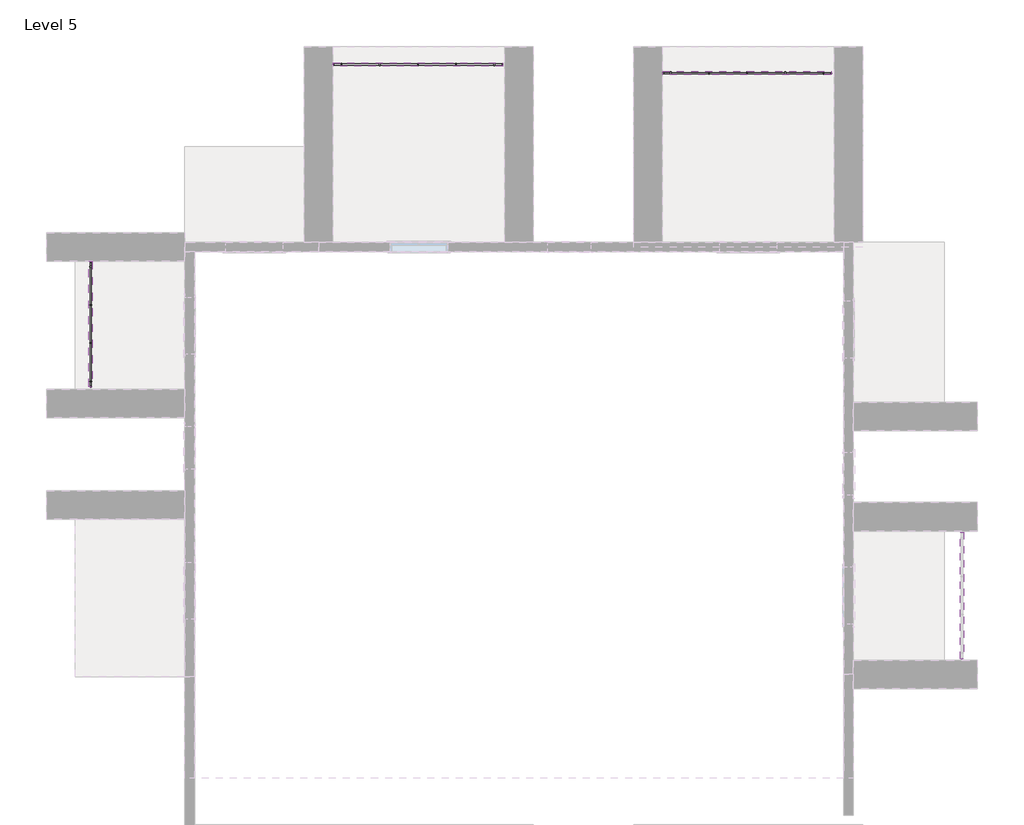
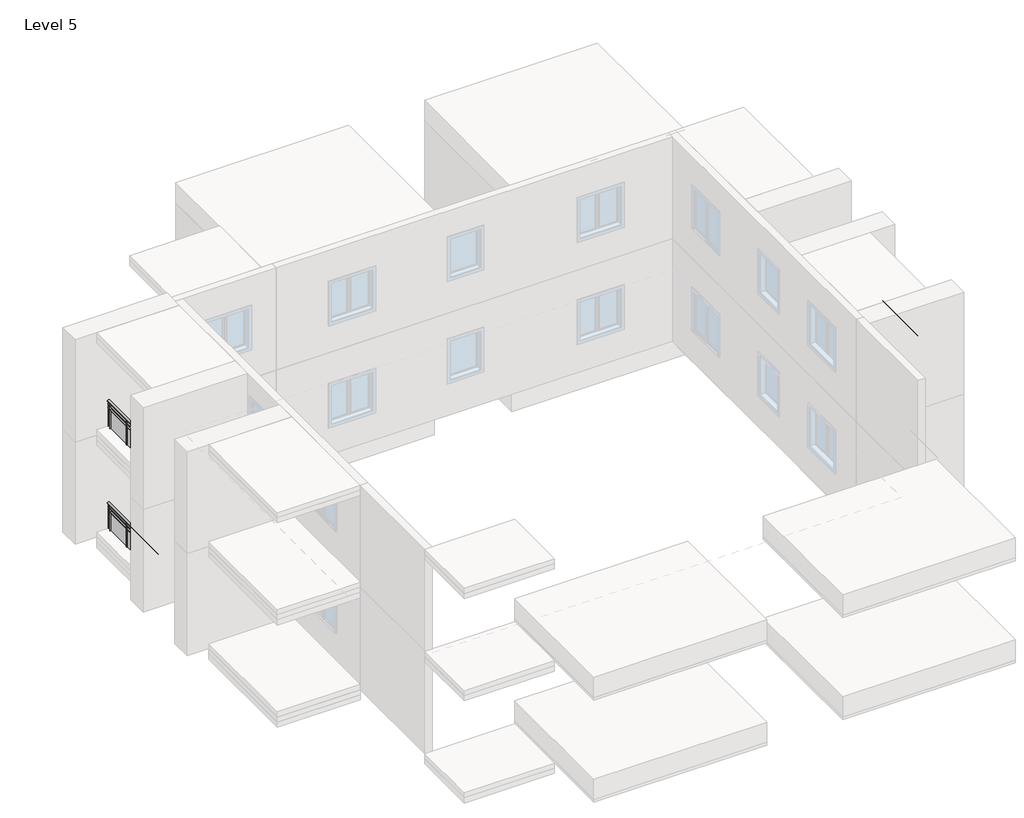
# One storey, part 4 of 4: 7 railings.
"""IFC4 building model written with IfcOpenShell, lengths in millimetres."""

from ifc_helpers import new_model, si_unit, point, frame, origin, place, context, project, spatial, polyline, ellipse_curve, trimmed, outline, extrude, element, save
from ifc_brep_helpers import plane_surface, extruded_surface, advanced_brep

model = new_model("IFC4")

# Units and contexts
model_context = context("Model", 3, world=origin())
ifc_project = project(units=[si_unit("LENGTHUNIT", "METRE", prefix="MILLI")], contexts=[model_context])

# Site, building, storey
site = spatial("IfcSite", under=ifc_project)
building = spatial("IfcBuilding", under=site)
storey = spatial("IfcBuildingStorey", under=building, Name="Level 5", Elevation=12192.0)

# Railings
placement = place(None, origin())
element("IfcRailing", 1, ObjectType="Glass Panel - Bottom Fill", at=placement, inside=storey, context=model_context, shape_type="SolidModel", body=[
    advanced_brep(
    [(-14351.1937431, 6115.813611, 13411.2), (-14427.3937431, 6115.813611, 13411.2), (-14351.1937431, 3448.813611, 13411.2), (-14427.3937431, 3448.813611, 13411.2)],
    [
        (0, 1, ellipse_curve(frame((-14389.2937431, 6115.813611, 13411.2), z_axis=(0.0, 1.0, 0.0), x_axis=(-1.0, 0.0, 0.0)), 38.1, 28.575)),
        (1, 0, ellipse_curve(frame((-14389.2937431, 6115.813611, 13411.2), z_axis=(0.0, 1.0, 0.0), x_axis=(-1.0, 0.0, 0.0)), 38.1, 28.575)),
        (2, 3, ellipse_curve(frame((-14389.2937431, 3448.813611, 13411.2), z_axis=(0.0, -1.0, 0.0), x_axis=(-1.0, 0.0, 0.0)), 38.1, 28.575)),
        (3, 2, ellipse_curve(frame((-14389.2937431, 3448.813611, 13411.2), z_axis=(0.0, -1.0, 0.0), x_axis=(-1.0, 0.0, 0.0)), 38.1, 28.575)),
        (0, 2),
        (3, 1),
    ],
    [
        plane_surface(frame((-14389.2937431, 6115.813611, 13411.2), z_axis=(0.0, 1.0, 0.0), x_axis=(0.0, 0.0, -1.0))),
        plane_surface(frame((-14389.2937431, 3448.813611, 13411.2), z_axis=(0.0, -1.0, 0.0), x_axis=(0.0, 0.0, -1.0))),
        extruded_surface(trimmed(ellipse_curve(frame((-14389.2937431, 3448.813611, 13411.2), z_axis=(0.0, 1.0, 0.0), x_axis=(-1.0, 0.0, 0.0)), 38.1, 28.575), [point((-14351.1937431, 3448.813611, 13411.2))], [point((-14427.3937431, 3448.813611, 13411.2))], True, "CARTESIAN"), (0.0, 2666.9999999999995, 0.0), 2666.9999999999995),
        extruded_surface(trimmed(ellipse_curve(frame((-14389.2937431, 3448.813611, 13411.2), z_axis=(0.0, 1.0, 0.0), x_axis=(-1.0, 0.0, 0.0)), 38.1, 28.575), [point((-14427.3937431, 3448.813611, 13411.2))], [point((-14351.1937431, 3448.813611, 13411.2))], True, "CARTESIAN"), (0.0, 2666.9999999999995, 0.0), 2666.9999999999995),
    ],
    [
        (0, [[1, 2]]),
        (1, [[3, 4]]),
        (2, [[-1, 5, -4, 6]]),
        (3, [[-2, -6, -3, -5]]),
    ],
),
    extrude(outline(polyline([(-14401.9937431, 6115.813611), (-14376.5937431, 6115.813611), (-14376.5937431, 3448.813611), (-14401.9937431, 3448.813611), (-14401.9937431, 6115.813611)])), frame((0.0, 0.0, 13296.9), z_axis=(0.0, 0.0, 1.0), x_axis=(1.0, 0.0, 0.0)), (0.0, 0.0, 1.0), 25.4),
    extrude(outline(polyline([(-14401.9937431, 6115.813611), (-14376.5937431, 6115.813611), (-14376.5937431, 3448.813611), (-14401.9937431, 3448.813611), (-14401.9937431, 6115.813611)])), frame((0.0, 0.0, 13195.3), z_axis=(0.0, 0.0, 1.0), x_axis=(1.0, 0.0, 0.0)), (0.0, 0.0, 1.0), 25.4),
    extrude(outline(polyline([(-14414.6937431, 3569.463611), (-14363.8937431, 3569.463611), (-14363.8937431, 3556.763611), (-14414.6937431, 3556.763611), (-14414.6937431, 3569.463611)])), frame((0.0, 0.0, 12496.8), z_axis=(0.0, 0.0, 1.0), x_axis=(1.0, 0.0, 0.0)), (0.0, 0.0, 1.0), 885.6788223),
    extrude(outline(polyline([(-14382.7585861, 4375.913611), (-14382.7585861, 3563.113611), (-14389.1085861, 3563.113611), (-14389.1085861, 4375.913611), (-14382.7585861, 4375.913611)])), frame((0.0, 0.0, 12598.4), z_axis=(0.0, 0.0, 1.0), x_axis=(1.0, 0.0, 0.0)), (0.0, 0.0, 1.0), 596.9),
    extrude(outline(polyline([(-14414.6937431, 4382.263611), (-14363.8937431, 4382.263611), (-14363.8937431, 4369.563611), (-14414.6937431, 4369.563611), (-14414.6937431, 4382.263611)])), frame((0.0, 0.0, 12496.8), z_axis=(0.0, 0.0, 1.0), x_axis=(1.0, 0.0, 0.0)), (0.0, 0.0, 1.0), 885.6788223),
    extrude(outline(polyline([(-14382.7585861, 5188.713611), (-14382.7585861, 4375.913611), (-14389.1085861, 4375.913611), (-14389.1085861, 5188.713611), (-14382.7585861, 5188.713611)])), frame((0.0, 0.0, 12598.4), z_axis=(0.0, 0.0, 1.0), x_axis=(1.0, 0.0, 0.0)), (0.0, 0.0, 1.0), 596.9),
    extrude(outline(polyline([(-14414.6937431, 5195.063611), (-14363.8937431, 5195.063611), (-14363.8937431, 5182.363611), (-14414.6937431, 5182.363611), (-14414.6937431, 5195.063611)])), frame((0.0, 0.0, 12496.8), z_axis=(0.0, 0.0, 1.0), x_axis=(1.0, 0.0, 0.0)), (0.0, 0.0, 1.0), 885.6788223),
    extrude(outline(polyline([(-14382.7585861, 6001.513611), (-14382.7585861, 5188.713611), (-14389.1085861, 5188.713611), (-14389.1085861, 6001.513611), (-14382.7585861, 6001.513611)])), frame((0.0, 0.0, 12598.4), z_axis=(0.0, 0.0, 1.0), x_axis=(1.0, 0.0, 0.0)), (0.0, 0.0, 1.0), 596.9),
    extrude(outline(polyline([(-14414.6937431, 6007.863611), (-14363.8937431, 6007.863611), (-14363.8937431, 5995.163611), (-14414.6937431, 5995.163611), (-14414.6937431, 6007.863611)])), frame((0.0, 0.0, 12496.8), z_axis=(0.0, 0.0, 1.0), x_axis=(1.0, 0.0, 0.0)), (0.0, 0.0, 1.0), 885.6788223),
    extrude(outline(polyline([(-14398.8187431, 3461.513611), (-14379.7687431, 3461.513611), (-14379.7687431, 3442.463611), (-14398.8187431, 3442.463611), (-14398.8187431, 3461.513611)])), frame((0.0, 0.0, 12496.8), z_axis=(0.0, 0.0, 1.0), x_axis=(1.0, 0.0, 0.0)), (0.0, 0.0, 1.0), 885.6788223),
    extrude(outline(polyline([(-14398.8187431, 6122.163611), (-14379.7687431, 6122.163611), (-14379.7687431, 6103.113611), (-14398.8187431, 6103.113611), (-14398.8187431, 6122.163611)])), frame((0.0, 0.0, 12496.8), z_axis=(0.0, 0.0, 1.0), x_axis=(1.0, 0.0, 0.0)), (0.0, 0.0, 1.0), 885.6788223),
])
element("IfcRailing", 2, ObjectType="Glass Panel - Bottom Fill", at=placement, inside=storey, context=model_context, shape_type="SolidModel", body=[
    advanced_brep(
    [(-9229.0758442, 10344.5205237, 13411.2), (-9229.0758442, 10268.3205237, 13411.2), (-5622.2758442, 10344.5205237, 13411.2), (-5622.2758442, 10268.3205237, 13411.2)],
    [
        (0, 1, ellipse_curve(frame((-9229.0758442, 10306.4205237, 13411.2), z_axis=(-1.0, 0.0, 0.0), x_axis=(0.0, -1.0, 0.0)), 38.1, 28.575)),
        (1, 0, ellipse_curve(frame((-9229.0758442, 10306.4205237, 13411.2), z_axis=(-1.0, 0.0, 0.0), x_axis=(0.0, -1.0, 0.0)), 38.1, 28.575)),
        (2, 3, ellipse_curve(frame((-5622.2758442, 10306.4205237, 13411.2), z_axis=(1.0, 0.0, 0.0), x_axis=(0.0, -1.0, 0.0)), 38.1, 28.575)),
        (3, 2, ellipse_curve(frame((-5622.2758442, 10306.4205237, 13411.2), z_axis=(1.0, 0.0, 0.0), x_axis=(0.0, -1.0, 0.0)), 38.1, 28.575)),
        (0, 2),
        (3, 1),
    ],
    [
        plane_surface(frame((-9229.0758442, 10306.4205237, 13411.2), z_axis=(-1.0, 0.0, 0.0), x_axis=(0.0, 1.0, 0.0))),
        plane_surface(frame((-5622.2758442, 10306.4205237, 13411.2), z_axis=(1.0, 0.0, 0.0), x_axis=(0.0, 1.0, 0.0))),
        extruded_surface(trimmed(ellipse_curve(frame((-5622.2758442, 10306.4205237, 13411.2), z_axis=(-1.0, 0.0, 0.0), x_axis=(0.0, -1.0, 0.0)), 38.1, 28.575), [point((-5622.2758442, 10344.5205237, 13411.2))], [point((-5622.2758442, 10268.3205237, 13411.2))], True, "CARTESIAN"), (-3606.8, 0.0, 0.0), 3606.8),
        extruded_surface(trimmed(ellipse_curve(frame((-5622.2758442, 10306.4205237, 13411.2), z_axis=(-1.0, 0.0, 0.0), x_axis=(0.0, -1.0, 0.0)), 38.1, 28.575), [point((-5622.2758442, 10268.3205237, 13411.2))], [point((-5622.2758442, 10344.5205237, 13411.2))], True, "CARTESIAN"), (-3606.8, 0.0, 0.0), 3606.8),
    ],
    [
        (0, [[1, 2]]),
        (1, [[3, 4]]),
        (2, [[-1, 5, -4, 6]]),
        (3, [[-2, -6, -3, -5]]),
    ],
),
    extrude(outline(polyline([(-9229.0758442, 10293.7205237), (-9229.0758442, 10319.1205237), (-5622.2758442, 10319.1205237), (-5622.2758442, 10293.7205237), (-9229.0758442, 10293.7205237)])), frame((0.0, 0.0, 13296.9), z_axis=(0.0, 0.0, 1.0), x_axis=(1.0, 0.0, 0.0)), (0.0, 0.0, 1.0), 25.4),
    extrude(outline(polyline([(-9229.0758442, 10293.7205237), (-9229.0758442, 10319.1205237), (-5622.2758442, 10319.1205237), (-5622.2758442, 10293.7205237), (-9229.0758442, 10293.7205237)])), frame((0.0, 0.0, 13195.3), z_axis=(0.0, 0.0, 1.0), x_axis=(1.0, 0.0, 0.0)), (0.0, 0.0, 1.0), 25.4),
    extrude(outline(polyline([(-5806.4258442, 10281.0205237), (-5806.4258442, 10331.8205237), (-5793.7258442, 10331.8205237), (-5793.7258442, 10281.0205237), (-5806.4258442, 10281.0205237)])), frame((0.0, 0.0, 12496.8), z_axis=(0.0, 0.0, 1.0), x_axis=(1.0, 0.0, 0.0)), (0.0, 0.0, 1.0), 885.6788223),
    extrude(outline(polyline([(-6612.8758442, 10312.9556807), (-5800.0758442, 10312.9556807), (-5800.0758442, 10306.6056807), (-6612.8758442, 10306.6056807), (-6612.8758442, 10312.9556807)])), frame((0.0, 0.0, 12598.4), z_axis=(0.0, 0.0, 1.0), x_axis=(1.0, 0.0, 0.0)), (0.0, 0.0, 1.0), 596.9),
    extrude(outline(polyline([(-6619.2258442, 10281.0205237), (-6619.2258442, 10331.8205237), (-6606.5258442, 10331.8205237), (-6606.5258442, 10281.0205237), (-6619.2258442, 10281.0205237)])), frame((0.0, 0.0, 12496.8), z_axis=(0.0, 0.0, 1.0), x_axis=(1.0, 0.0, 0.0)), (0.0, 0.0, 1.0), 885.6788223),
    extrude(outline(polyline([(-7425.6758442, 10312.9556807), (-6612.8758442, 10312.9556807), (-6612.8758442, 10306.6056807), (-7425.6758442, 10306.6056807), (-7425.6758442, 10312.9556807)])), frame((0.0, 0.0, 12598.4), z_axis=(0.0, 0.0, 1.0), x_axis=(1.0, 0.0, 0.0)), (0.0, 0.0, 1.0), 596.9),
    extrude(outline(polyline([(-7432.0258442, 10281.0205237), (-7432.0258442, 10331.8205237), (-7419.3258442, 10331.8205237), (-7419.3258442, 10281.0205237), (-7432.0258442, 10281.0205237)])), frame((0.0, 0.0, 12496.8), z_axis=(0.0, 0.0, 1.0), x_axis=(1.0, 0.0, 0.0)), (0.0, 0.0, 1.0), 885.6788223),
    extrude(outline(polyline([(-8238.4758442, 10312.9556807), (-7425.6758442, 10312.9556807), (-7425.6758442, 10306.6056807), (-8238.4758442, 10306.6056807), (-8238.4758442, 10312.9556807)])), frame((0.0, 0.0, 12598.4), z_axis=(0.0, 0.0, 1.0), x_axis=(1.0, 0.0, 0.0)), (0.0, 0.0, 1.0), 596.9),
    extrude(outline(polyline([(-8244.8258442, 10281.0205237), (-8244.8258442, 10331.8205237), (-8232.1258442, 10331.8205237), (-8232.1258442, 10281.0205237), (-8244.8258442, 10281.0205237)])), frame((0.0, 0.0, 12496.8), z_axis=(0.0, 0.0, 1.0), x_axis=(1.0, 0.0, 0.0)), (0.0, 0.0, 1.0), 885.6788223),
    extrude(outline(polyline([(-9051.2758442, 10312.9556807), (-8238.4758442, 10312.9556807), (-8238.4758442, 10306.6056807), (-9051.2758442, 10306.6056807), (-9051.2758442, 10312.9556807)])), frame((0.0, 0.0, 12598.4), z_axis=(0.0, 0.0, 1.0), x_axis=(1.0, 0.0, 0.0)), (0.0, 0.0, 1.0), 596.9),
    extrude(outline(polyline([(-9057.6258442, 10281.0205237), (-9057.6258442, 10331.8205237), (-9044.9258442, 10331.8205237), (-9044.9258442, 10281.0205237), (-9057.6258442, 10281.0205237)])), frame((0.0, 0.0, 12496.8), z_axis=(0.0, 0.0, 1.0), x_axis=(1.0, 0.0, 0.0)), (0.0, 0.0, 1.0), 885.6788223),
    extrude(outline(polyline([(-5634.9758442, 10296.8955237), (-5634.9758442, 10315.9455237), (-5615.9258442, 10315.9455237), (-5615.9258442, 10296.8955237), (-5634.9758442, 10296.8955237)])), frame((0.0, 0.0, 12496.8), z_axis=(0.0, 0.0, 1.0), x_axis=(1.0, 0.0, 0.0)), (0.0, 0.0, 1.0), 885.6788223),
    extrude(outline(polyline([(-9235.4258442, 10296.8955237), (-9235.4258442, 10315.9455237), (-9216.3758442, 10315.9455237), (-9216.3758442, 10296.8955237), (-9235.4258442, 10296.8955237)])), frame((0.0, 0.0, 12496.8), z_axis=(0.0, 0.0, 1.0), x_axis=(1.0, 0.0, 0.0)), (0.0, 0.0, 1.0), 885.6788223),
])
element("IfcRailing", 3, ObjectType="Glass Panel - Bottom Fill", at=placement, inside=storey, context=model_context, shape_type="SolidModel", body=[
    advanced_brep(
    [(-2210.3891352, 10161.3373193, 13411.2), (-2210.3891352, 10085.1373193, 13411.2), (1371.0108648, 10161.3373193, 13411.2), (1371.0108648, 10085.1373193, 13411.2)],
    [
        (0, 1, ellipse_curve(frame((-2210.3891352, 10123.2373193, 13411.2), z_axis=(-1.0, 0.0, 0.0), x_axis=(0.0, -1.0, 0.0)), 38.1, 28.575)),
        (1, 0, ellipse_curve(frame((-2210.3891352, 10123.2373193, 13411.2), z_axis=(-1.0, 0.0, 0.0), x_axis=(0.0, -1.0, 0.0)), 38.1, 28.575)),
        (2, 3, ellipse_curve(frame((1371.0108648, 10123.2373193, 13411.2), z_axis=(1.0, 0.0, 0.0), x_axis=(0.0, -1.0, 0.0)), 38.1, 28.575)),
        (3, 2, ellipse_curve(frame((1371.0108648, 10123.2373193, 13411.2), z_axis=(1.0, 0.0, 0.0), x_axis=(0.0, -1.0, 0.0)), 38.1, 28.575)),
        (0, 2),
        (3, 1),
    ],
    [
        plane_surface(frame((-2210.3891352, 10123.2373193, 13411.2), z_axis=(-1.0, 0.0, 0.0), x_axis=(0.0, 1.0, 0.0))),
        plane_surface(frame((1371.0108648, 10123.2373193, 13411.2), z_axis=(1.0, 0.0, 0.0), x_axis=(0.0, 1.0, 0.0))),
        extruded_surface(trimmed(ellipse_curve(frame((1371.0108648, 10123.2373193, 13411.2), z_axis=(-1.0, 0.0, 0.0), x_axis=(0.0, -1.0, 0.0)), 38.1, 28.575), [point((1371.0108648, 10161.3373193, 13411.2))], [point((1371.0108648, 10085.1373193, 13411.2))], True, "CARTESIAN"), (-3581.4, 0.0, 0.0), 3581.4),
        extruded_surface(trimmed(ellipse_curve(frame((1371.0108648, 10123.2373193, 13411.2), z_axis=(-1.0, 0.0, 0.0), x_axis=(0.0, -1.0, 0.0)), 38.1, 28.575), [point((1371.0108648, 10085.1373193, 13411.2))], [point((1371.0108648, 10161.3373193, 13411.2))], True, "CARTESIAN"), (-3581.4, 0.0, 0.0), 3581.4),
    ],
    [
        (0, [[1, 2]]),
        (1, [[3, 4]]),
        (2, [[-1, 5, -4, 6]]),
        (3, [[-2, -6, -3, -5]]),
    ],
),
    extrude(outline(polyline([(-2210.3891352, 10110.5373193), (-2210.3891352, 10135.9373193), (1371.0108648, 10135.9373193), (1371.0108648, 10110.5373193), (-2210.3891352, 10110.5373193)])), frame((0.0, 0.0, 13296.9), z_axis=(0.0, 0.0, 1.0), x_axis=(1.0, 0.0, 0.0)), (0.0, 0.0, 1.0), 25.4),
    extrude(outline(polyline([(-2210.3891352, 10110.5373193), (-2210.3891352, 10135.9373193), (1371.0108648, 10135.9373193), (1371.0108648, 10110.5373193), (-2210.3891352, 10110.5373193)])), frame((0.0, 0.0, 13195.3), z_axis=(0.0, 0.0, 1.0), x_axis=(1.0, 0.0, 0.0)), (0.0, 0.0, 1.0), 25.4),
    extrude(outline(polyline([(1199.5608648, 10097.8373193), (1199.5608648, 10148.6373193), (1212.2608648, 10148.6373193), (1212.2608648, 10097.8373193), (1199.5608648, 10097.8373193)])), frame((0.0, 0.0, 12496.8), z_axis=(0.0, 0.0, 1.0), x_axis=(1.0, 0.0, 0.0)), (0.0, 0.0, 1.0), 885.6788223),
    extrude(outline(polyline([(393.1108648, 10129.7724763), (1205.9108648, 10129.7724763), (1205.9108648, 10123.4224763), (393.1108648, 10123.4224763), (393.1108648, 10129.7724763)])), frame((0.0, 0.0, 12598.4), z_axis=(0.0, 0.0, 1.0), x_axis=(1.0, 0.0, 0.0)), (0.0, 0.0, 1.0), 596.9),
    extrude(outline(polyline([(386.7608648, 10097.8373193), (386.7608648, 10148.6373193), (399.4608648, 10148.6373193), (399.4608648, 10097.8373193), (386.7608648, 10097.8373193)])), frame((0.0, 0.0, 12496.8), z_axis=(0.0, 0.0, 1.0), x_axis=(1.0, 0.0, 0.0)), (0.0, 0.0, 1.0), 885.6788223),
    extrude(outline(polyline([(-419.6891352, 10129.7724763), (393.1108648, 10129.7724763), (393.1108648, 10123.4224763), (-419.6891352, 10123.4224763), (-419.6891352, 10129.7724763)])), frame((0.0, 0.0, 12598.4), z_axis=(0.0, 0.0, 1.0), x_axis=(1.0, 0.0, 0.0)), (0.0, 0.0, 1.0), 596.9),
    extrude(outline(polyline([(-426.0391352, 10097.8373193), (-426.0391352, 10148.6373193), (-413.3391352, 10148.6373193), (-413.3391352, 10097.8373193), (-426.0391352, 10097.8373193)])), frame((0.0, 0.0, 12496.8), z_axis=(0.0, 0.0, 1.0), x_axis=(1.0, 0.0, 0.0)), (0.0, 0.0, 1.0), 885.6788223),
    extrude(outline(polyline([(-1232.4891352, 10129.7724763), (-419.6891352, 10129.7724763), (-419.6891352, 10123.4224763), (-1232.4891352, 10123.4224763), (-1232.4891352, 10129.7724763)])), frame((0.0, 0.0, 12598.4), z_axis=(0.0, 0.0, 1.0), x_axis=(1.0, 0.0, 0.0)), (0.0, 0.0, 1.0), 596.9),
    extrude(outline(polyline([(-1238.8391352, 10097.8373193), (-1238.8391352, 10148.6373193), (-1226.1391352, 10148.6373193), (-1226.1391352, 10097.8373193), (-1238.8391352, 10097.8373193)])), frame((0.0, 0.0, 12496.8), z_axis=(0.0, 0.0, 1.0), x_axis=(1.0, 0.0, 0.0)), (0.0, 0.0, 1.0), 885.6788223),
    extrude(outline(polyline([(-2045.2891352, 10129.7724763), (-1232.4891352, 10129.7724763), (-1232.4891352, 10123.4224763), (-2045.2891352, 10123.4224763), (-2045.2891352, 10129.7724763)])), frame((0.0, 0.0, 12598.4), z_axis=(0.0, 0.0, 1.0), x_axis=(1.0, 0.0, 0.0)), (0.0, 0.0, 1.0), 596.9),
    extrude(outline(polyline([(-2051.6391352, 10097.8373193), (-2051.6391352, 10148.6373193), (-2038.9391352, 10148.6373193), (-2038.9391352, 10097.8373193), (-2051.6391352, 10097.8373193)])), frame((0.0, 0.0, 12496.8), z_axis=(0.0, 0.0, 1.0), x_axis=(1.0, 0.0, 0.0)), (0.0, 0.0, 1.0), 885.6788223),
    extrude(outline(polyline([(1358.3108648, 10113.7123193), (1358.3108648, 10132.7623193), (1377.3608648, 10132.7623193), (1377.3608648, 10113.7123193), (1358.3108648, 10113.7123193)])), frame((0.0, 0.0, 12496.8), z_axis=(0.0, 0.0, 1.0), x_axis=(1.0, 0.0, 0.0)), (0.0, 0.0, 1.0), 885.6788223),
    extrude(outline(polyline([(-2216.7391352, 10113.7123193), (-2216.7391352, 10132.7623193), (-2197.6891352, 10132.7623193), (-2197.6891352, 10113.7123193), (-2216.7391352, 10113.7123193)])), frame((0.0, 0.0, 12496.8), z_axis=(0.0, 0.0, 1.0), x_axis=(1.0, 0.0, 0.0)), (0.0, 0.0, 1.0), 885.6788223),
])
element("IfcRailing", 4, ObjectType="Glass Panel - Bottom Fill", at=placement, inside=storey, context=model_context, shape_type="SolidModel", body=[
    advanced_brep(
    [(-14351.1937431, 6115.813611, 16459.2), (-14427.3937431, 6115.813611, 16459.2), (-14351.1937431, 3448.813611, 16459.2), (-14427.3937431, 3448.813611, 16459.2)],
    [
        (0, 1, ellipse_curve(frame((-14389.2937431, 6115.813611, 16459.2), z_axis=(0.0, 1.0, 0.0), x_axis=(-1.0, 0.0, 0.0)), 38.1, 28.575)),
        (1, 0, ellipse_curve(frame((-14389.2937431, 6115.813611, 16459.2), z_axis=(0.0, 1.0, 0.0), x_axis=(-1.0, 0.0, 0.0)), 38.1, 28.575)),
        (2, 3, ellipse_curve(frame((-14389.2937431, 3448.813611, 16459.2), z_axis=(0.0, -1.0, 0.0), x_axis=(-1.0, 0.0, 0.0)), 38.1, 28.575)),
        (3, 2, ellipse_curve(frame((-14389.2937431, 3448.813611, 16459.2), z_axis=(0.0, -1.0, 0.0), x_axis=(-1.0, 0.0, 0.0)), 38.1, 28.575)),
        (0, 2),
        (3, 1),
    ],
    [
        plane_surface(frame((-14389.2937431, 6115.813611, 16459.2), z_axis=(0.0, 1.0, 0.0), x_axis=(0.0, 0.0, -1.0))),
        plane_surface(frame((-14389.2937431, 3448.813611, 16459.2), z_axis=(0.0, -1.0, 0.0), x_axis=(0.0, 0.0, -1.0))),
        extruded_surface(trimmed(ellipse_curve(frame((-14389.2937431, 3448.813611, 16459.2), z_axis=(0.0, 1.0, 0.0), x_axis=(-1.0, 0.0, 0.0)), 38.1, 28.575), [point((-14351.1937431, 3448.813611, 16459.2))], [point((-14427.3937431, 3448.813611, 16459.2))], True, "CARTESIAN"), (0.0, 2666.9999999999995, 0.0), 2666.9999999999995),
        extruded_surface(trimmed(ellipse_curve(frame((-14389.2937431, 3448.813611, 16459.2), z_axis=(0.0, 1.0, 0.0), x_axis=(-1.0, 0.0, 0.0)), 38.1, 28.575), [point((-14427.3937431, 3448.813611, 16459.2))], [point((-14351.1937431, 3448.813611, 16459.2))], True, "CARTESIAN"), (0.0, 2666.9999999999995, 0.0), 2666.9999999999995),
    ],
    [
        (0, [[1, 2]]),
        (1, [[3, 4]]),
        (2, [[-1, 5, -4, 6]]),
        (3, [[-2, -6, -3, -5]]),
    ],
),
    extrude(outline(polyline([(-14401.9937431, 6115.813611), (-14376.5937431, 6115.813611), (-14376.5937431, 3448.813611), (-14401.9937431, 3448.813611), (-14401.9937431, 6115.813611)])), frame((0.0, 0.0, 16344.9), z_axis=(0.0, 0.0, 1.0), x_axis=(1.0, 0.0, 0.0)), (0.0, 0.0, 1.0), 25.4),
    extrude(outline(polyline([(-14401.9937431, 6115.813611), (-14376.5937431, 6115.813611), (-14376.5937431, 3448.813611), (-14401.9937431, 3448.813611), (-14401.9937431, 6115.813611)])), frame((0.0, 0.0, 16243.3), z_axis=(0.0, 0.0, 1.0), x_axis=(1.0, 0.0, 0.0)), (0.0, 0.0, 1.0), 25.4),
    extrude(outline(polyline([(-14414.6937431, 3569.463611), (-14363.8937431, 3569.463611), (-14363.8937431, 3556.763611), (-14414.6937431, 3556.763611), (-14414.6937431, 3569.463611)])), frame((0.0, 0.0, 15544.8), z_axis=(0.0, 0.0, 1.0), x_axis=(1.0, 0.0, 0.0)), (0.0, 0.0, 1.0), 885.6788223),
    extrude(outline(polyline([(-14382.7585861, 4375.913611), (-14382.7585861, 3563.113611), (-14389.1085861, 3563.113611), (-14389.1085861, 4375.913611), (-14382.7585861, 4375.913611)])), frame((0.0, 0.0, 15646.4), z_axis=(0.0, 0.0, 1.0), x_axis=(1.0, 0.0, 0.0)), (0.0, 0.0, 1.0), 596.9),
    extrude(outline(polyline([(-14414.6937431, 4382.263611), (-14363.8937431, 4382.263611), (-14363.8937431, 4369.563611), (-14414.6937431, 4369.563611), (-14414.6937431, 4382.263611)])), frame((0.0, 0.0, 15544.8), z_axis=(0.0, 0.0, 1.0), x_axis=(1.0, 0.0, 0.0)), (0.0, 0.0, 1.0), 885.6788223),
    extrude(outline(polyline([(-14382.7585861, 5188.713611), (-14382.7585861, 4375.913611), (-14389.1085861, 4375.913611), (-14389.1085861, 5188.713611), (-14382.7585861, 5188.713611)])), frame((0.0, 0.0, 15646.4), z_axis=(0.0, 0.0, 1.0), x_axis=(1.0, 0.0, 0.0)), (0.0, 0.0, 1.0), 596.9),
    extrude(outline(polyline([(-14414.6937431, 5195.063611), (-14363.8937431, 5195.063611), (-14363.8937431, 5182.363611), (-14414.6937431, 5182.363611), (-14414.6937431, 5195.063611)])), frame((0.0, 0.0, 15544.8), z_axis=(0.0, 0.0, 1.0), x_axis=(1.0, 0.0, 0.0)), (0.0, 0.0, 1.0), 885.6788223),
    extrude(outline(polyline([(-14382.7585861, 6001.513611), (-14382.7585861, 5188.713611), (-14389.1085861, 5188.713611), (-14389.1085861, 6001.513611), (-14382.7585861, 6001.513611)])), frame((0.0, 0.0, 15646.4), z_axis=(0.0, 0.0, 1.0), x_axis=(1.0, 0.0, 0.0)), (0.0, 0.0, 1.0), 596.9),
    extrude(outline(polyline([(-14414.6937431, 6007.863611), (-14363.8937431, 6007.863611), (-14363.8937431, 5995.163611), (-14414.6937431, 5995.163611), (-14414.6937431, 6007.863611)])), frame((0.0, 0.0, 15544.8), z_axis=(0.0, 0.0, 1.0), x_axis=(1.0, 0.0, 0.0)), (0.0, 0.0, 1.0), 885.6788223),
    extrude(outline(polyline([(-14398.8187431, 3461.513611), (-14379.7687431, 3461.513611), (-14379.7687431, 3442.463611), (-14398.8187431, 3442.463611), (-14398.8187431, 3461.513611)])), frame((0.0, 0.0, 15544.8), z_axis=(0.0, 0.0, 1.0), x_axis=(1.0, 0.0, 0.0)), (0.0, 0.0, 1.0), 885.6788223),
    extrude(outline(polyline([(-14398.8187431, 6122.163611), (-14379.7687431, 6122.163611), (-14379.7687431, 6103.113611), (-14398.8187431, 6103.113611), (-14398.8187431, 6122.163611)])), frame((0.0, 0.0, 15544.8), z_axis=(0.0, 0.0, 1.0), x_axis=(1.0, 0.0, 0.0)), (0.0, 0.0, 1.0), 885.6788223),
])
element("IfcRailing", 5, ObjectType="Glass Panel - Bottom Fill", at=placement, inside=storey, context=model_context, shape_type="SolidModel", body=[
    advanced_brep(
    [(-9229.0758442, 10344.5205237, 16459.2), (-9229.0758442, 10268.3205237, 16459.2), (-5622.2758442, 10344.5205237, 16459.2), (-5622.2758442, 10268.3205237, 16459.2)],
    [
        (0, 1, ellipse_curve(frame((-9229.0758442, 10306.4205237, 16459.2), z_axis=(-1.0, 0.0, 0.0), x_axis=(0.0, -1.0, 0.0)), 38.1, 28.575)),
        (1, 0, ellipse_curve(frame((-9229.0758442, 10306.4205237, 16459.2), z_axis=(-1.0, 0.0, 0.0), x_axis=(0.0, -1.0, 0.0)), 38.1, 28.575)),
        (2, 3, ellipse_curve(frame((-5622.2758442, 10306.4205237, 16459.2), z_axis=(1.0, 0.0, 0.0), x_axis=(0.0, -1.0, 0.0)), 38.1, 28.575)),
        (3, 2, ellipse_curve(frame((-5622.2758442, 10306.4205237, 16459.2), z_axis=(1.0, 0.0, 0.0), x_axis=(0.0, -1.0, 0.0)), 38.1, 28.575)),
        (0, 2),
        (3, 1),
    ],
    [
        plane_surface(frame((-9229.0758442, 10306.4205237, 16459.2), z_axis=(-1.0, 0.0, 0.0), x_axis=(0.0, 1.0, 0.0))),
        plane_surface(frame((-5622.2758442, 10306.4205237, 16459.2), z_axis=(1.0, 0.0, 0.0), x_axis=(0.0, 1.0, 0.0))),
        extruded_surface(trimmed(ellipse_curve(frame((-5622.2758442, 10306.4205237, 16459.2), z_axis=(-1.0, 0.0, 0.0), x_axis=(0.0, -1.0, 0.0)), 38.1, 28.575), [point((-5622.2758442, 10344.5205237, 16459.2))], [point((-5622.2758442, 10268.3205237, 16459.2))], True, "CARTESIAN"), (-3606.8, 0.0, 0.0), 3606.8),
        extruded_surface(trimmed(ellipse_curve(frame((-5622.2758442, 10306.4205237, 16459.2), z_axis=(-1.0, 0.0, 0.0), x_axis=(0.0, -1.0, 0.0)), 38.1, 28.575), [point((-5622.2758442, 10268.3205237, 16459.2))], [point((-5622.2758442, 10344.5205237, 16459.2))], True, "CARTESIAN"), (-3606.8, 0.0, 0.0), 3606.8),
    ],
    [
        (0, [[1, 2]]),
        (1, [[3, 4]]),
        (2, [[-1, 5, -4, 6]]),
        (3, [[-2, -6, -3, -5]]),
    ],
),
    extrude(outline(polyline([(-9229.0758442, 10293.7205237), (-9229.0758442, 10319.1205237), (-5622.2758442, 10319.1205237), (-5622.2758442, 10293.7205237), (-9229.0758442, 10293.7205237)])), frame((0.0, 0.0, 16344.9), z_axis=(0.0, 0.0, 1.0), x_axis=(1.0, 0.0, 0.0)), (0.0, 0.0, 1.0), 25.4),
    extrude(outline(polyline([(-9229.0758442, 10293.7205237), (-9229.0758442, 10319.1205237), (-5622.2758442, 10319.1205237), (-5622.2758442, 10293.7205237), (-9229.0758442, 10293.7205237)])), frame((0.0, 0.0, 16243.3), z_axis=(0.0, 0.0, 1.0), x_axis=(1.0, 0.0, 0.0)), (0.0, 0.0, 1.0), 25.4),
    extrude(outline(polyline([(-5806.4258442, 10281.0205237), (-5806.4258442, 10331.8205237), (-5793.7258442, 10331.8205237), (-5793.7258442, 10281.0205237), (-5806.4258442, 10281.0205237)])), frame((0.0, 0.0, 15544.8), z_axis=(0.0, 0.0, 1.0), x_axis=(1.0, 0.0, 0.0)), (0.0, 0.0, 1.0), 885.6788223),
    extrude(outline(polyline([(-6612.8758442, 10312.9556807), (-5800.0758442, 10312.9556807), (-5800.0758442, 10306.6056807), (-6612.8758442, 10306.6056807), (-6612.8758442, 10312.9556807)])), frame((0.0, 0.0, 15646.4), z_axis=(0.0, 0.0, 1.0), x_axis=(1.0, 0.0, 0.0)), (0.0, 0.0, 1.0), 596.9),
    extrude(outline(polyline([(-6619.2258442, 10281.0205237), (-6619.2258442, 10331.8205237), (-6606.5258442, 10331.8205237), (-6606.5258442, 10281.0205237), (-6619.2258442, 10281.0205237)])), frame((0.0, 0.0, 15544.8), z_axis=(0.0, 0.0, 1.0), x_axis=(1.0, 0.0, 0.0)), (0.0, 0.0, 1.0), 885.6788223),
    extrude(outline(polyline([(-7425.6758442, 10312.9556807), (-6612.8758442, 10312.9556807), (-6612.8758442, 10306.6056807), (-7425.6758442, 10306.6056807), (-7425.6758442, 10312.9556807)])), frame((0.0, 0.0, 15646.4), z_axis=(0.0, 0.0, 1.0), x_axis=(1.0, 0.0, 0.0)), (0.0, 0.0, 1.0), 596.9),
    extrude(outline(polyline([(-7432.0258442, 10281.0205237), (-7432.0258442, 10331.8205237), (-7419.3258442, 10331.8205237), (-7419.3258442, 10281.0205237), (-7432.0258442, 10281.0205237)])), frame((0.0, 0.0, 15544.8), z_axis=(0.0, 0.0, 1.0), x_axis=(1.0, 0.0, 0.0)), (0.0, 0.0, 1.0), 885.6788223),
    extrude(outline(polyline([(-8238.4758442, 10312.9556807), (-7425.6758442, 10312.9556807), (-7425.6758442, 10306.6056807), (-8238.4758442, 10306.6056807), (-8238.4758442, 10312.9556807)])), frame((0.0, 0.0, 15646.4), z_axis=(0.0, 0.0, 1.0), x_axis=(1.0, 0.0, 0.0)), (0.0, 0.0, 1.0), 596.9),
    extrude(outline(polyline([(-8244.8258442, 10281.0205237), (-8244.8258442, 10331.8205237), (-8232.1258442, 10331.8205237), (-8232.1258442, 10281.0205237), (-8244.8258442, 10281.0205237)])), frame((0.0, 0.0, 15544.8), z_axis=(0.0, 0.0, 1.0), x_axis=(1.0, 0.0, 0.0)), (0.0, 0.0, 1.0), 885.6788223),
    extrude(outline(polyline([(-9051.2758442, 10312.9556807), (-8238.4758442, 10312.9556807), (-8238.4758442, 10306.6056807), (-9051.2758442, 10306.6056807), (-9051.2758442, 10312.9556807)])), frame((0.0, 0.0, 15646.4), z_axis=(0.0, 0.0, 1.0), x_axis=(1.0, 0.0, 0.0)), (0.0, 0.0, 1.0), 596.9),
    extrude(outline(polyline([(-9057.6258442, 10281.0205237), (-9057.6258442, 10331.8205237), (-9044.9258442, 10331.8205237), (-9044.9258442, 10281.0205237), (-9057.6258442, 10281.0205237)])), frame((0.0, 0.0, 15544.8), z_axis=(0.0, 0.0, 1.0), x_axis=(1.0, 0.0, 0.0)), (0.0, 0.0, 1.0), 885.6788223),
    extrude(outline(polyline([(-5634.9758442, 10296.8955237), (-5634.9758442, 10315.9455237), (-5615.9258442, 10315.9455237), (-5615.9258442, 10296.8955237), (-5634.9758442, 10296.8955237)])), frame((0.0, 0.0, 15544.8), z_axis=(0.0, 0.0, 1.0), x_axis=(1.0, 0.0, 0.0)), (0.0, 0.0, 1.0), 885.6788223),
    extrude(outline(polyline([(-9235.4258442, 10296.8955237), (-9235.4258442, 10315.9455237), (-9216.3758442, 10315.9455237), (-9216.3758442, 10296.8955237), (-9235.4258442, 10296.8955237)])), frame((0.0, 0.0, 15544.8), z_axis=(0.0, 0.0, 1.0), x_axis=(1.0, 0.0, 0.0)), (0.0, 0.0, 1.0), 885.6788223),
])
element("IfcRailing", 6, ObjectType="Glass Panel - Bottom Fill", at=placement, inside=storey, context=model_context, shape_type="SolidModel", body=[
    advanced_brep(
    [(-2210.3891352, 10161.3373193, 16459.2), (-2210.3891352, 10085.1373193, 16459.2), (1371.0108648, 10161.3373193, 16459.2), (1371.0108648, 10085.1373193, 16459.2)],
    [
        (0, 1, ellipse_curve(frame((-2210.3891352, 10123.2373193, 16459.2), z_axis=(-1.0, 0.0, 0.0), x_axis=(0.0, -1.0, 0.0)), 38.1, 28.575)),
        (1, 0, ellipse_curve(frame((-2210.3891352, 10123.2373193, 16459.2), z_axis=(-1.0, 0.0, 0.0), x_axis=(0.0, -1.0, 0.0)), 38.1, 28.575)),
        (2, 3, ellipse_curve(frame((1371.0108648, 10123.2373193, 16459.2), z_axis=(1.0, 0.0, 0.0), x_axis=(0.0, -1.0, 0.0)), 38.1, 28.575)),
        (3, 2, ellipse_curve(frame((1371.0108648, 10123.2373193, 16459.2), z_axis=(1.0, 0.0, 0.0), x_axis=(0.0, -1.0, 0.0)), 38.1, 28.575)),
        (0, 2),
        (3, 1),
    ],
    [
        plane_surface(frame((-2210.3891352, 10123.2373193, 16459.2), z_axis=(-1.0, 0.0, 0.0), x_axis=(0.0, 1.0, 0.0))),
        plane_surface(frame((1371.0108648, 10123.2373193, 16459.2), z_axis=(1.0, 0.0, 0.0), x_axis=(0.0, 1.0, 0.0))),
        extruded_surface(trimmed(ellipse_curve(frame((1371.0108648, 10123.2373193, 16459.2), z_axis=(-1.0, 0.0, 0.0), x_axis=(0.0, -1.0, 0.0)), 38.1, 28.575), [point((1371.0108648, 10161.3373193, 16459.2))], [point((1371.0108648, 10085.1373193, 16459.2))], True, "CARTESIAN"), (-3581.4, 0.0, 0.0), 3581.4),
        extruded_surface(trimmed(ellipse_curve(frame((1371.0108648, 10123.2373193, 16459.2), z_axis=(-1.0, 0.0, 0.0), x_axis=(0.0, -1.0, 0.0)), 38.1, 28.575), [point((1371.0108648, 10085.1373193, 16459.2))], [point((1371.0108648, 10161.3373193, 16459.2))], True, "CARTESIAN"), (-3581.4, 0.0, 0.0), 3581.4),
    ],
    [
        (0, [[1, 2]]),
        (1, [[3, 4]]),
        (2, [[-1, 5, -4, 6]]),
        (3, [[-2, -6, -3, -5]]),
    ],
),
    extrude(outline(polyline([(-2210.3891352, 10110.5373193), (-2210.3891352, 10135.9373193), (1371.0108648, 10135.9373193), (1371.0108648, 10110.5373193), (-2210.3891352, 10110.5373193)])), frame((0.0, 0.0, 16344.9), z_axis=(0.0, 0.0, 1.0), x_axis=(1.0, 0.0, 0.0)), (0.0, 0.0, 1.0), 25.4),
    extrude(outline(polyline([(-2210.3891352, 10110.5373193), (-2210.3891352, 10135.9373193), (1371.0108648, 10135.9373193), (1371.0108648, 10110.5373193), (-2210.3891352, 10110.5373193)])), frame((0.0, 0.0, 16243.3), z_axis=(0.0, 0.0, 1.0), x_axis=(1.0, 0.0, 0.0)), (0.0, 0.0, 1.0), 25.4),
    extrude(outline(polyline([(1199.5608648, 10097.8373193), (1199.5608648, 10148.6373193), (1212.2608648, 10148.6373193), (1212.2608648, 10097.8373193), (1199.5608648, 10097.8373193)])), frame((0.0, 0.0, 15544.8), z_axis=(0.0, 0.0, 1.0), x_axis=(1.0, 0.0, 0.0)), (0.0, 0.0, 1.0), 885.6788223),
    extrude(outline(polyline([(393.1108648, 10129.7724763), (1205.9108648, 10129.7724763), (1205.9108648, 10123.4224763), (393.1108648, 10123.4224763), (393.1108648, 10129.7724763)])), frame((0.0, 0.0, 15646.4), z_axis=(0.0, 0.0, 1.0), x_axis=(1.0, 0.0, 0.0)), (0.0, 0.0, 1.0), 596.9),
    extrude(outline(polyline([(386.7608648, 10097.8373193), (386.7608648, 10148.6373193), (399.4608648, 10148.6373193), (399.4608648, 10097.8373193), (386.7608648, 10097.8373193)])), frame((0.0, 0.0, 15544.8), z_axis=(0.0, 0.0, 1.0), x_axis=(1.0, 0.0, 0.0)), (0.0, 0.0, 1.0), 885.6788223),
    extrude(outline(polyline([(-419.6891352, 10129.7724763), (393.1108648, 10129.7724763), (393.1108648, 10123.4224763), (-419.6891352, 10123.4224763), (-419.6891352, 10129.7724763)])), frame((0.0, 0.0, 15646.4), z_axis=(0.0, 0.0, 1.0), x_axis=(1.0, 0.0, 0.0)), (0.0, 0.0, 1.0), 596.9),
    extrude(outline(polyline([(-426.0391352, 10097.8373193), (-426.0391352, 10148.6373193), (-413.3391352, 10148.6373193), (-413.3391352, 10097.8373193), (-426.0391352, 10097.8373193)])), frame((0.0, 0.0, 15544.8), z_axis=(0.0, 0.0, 1.0), x_axis=(1.0, 0.0, 0.0)), (0.0, 0.0, 1.0), 885.6788223),
    extrude(outline(polyline([(-1232.4891352, 10129.7724763), (-419.6891352, 10129.7724763), (-419.6891352, 10123.4224763), (-1232.4891352, 10123.4224763), (-1232.4891352, 10129.7724763)])), frame((0.0, 0.0, 15646.4), z_axis=(0.0, 0.0, 1.0), x_axis=(1.0, 0.0, 0.0)), (0.0, 0.0, 1.0), 596.9),
    extrude(outline(polyline([(-1238.8391352, 10097.8373193), (-1238.8391352, 10148.6373193), (-1226.1391352, 10148.6373193), (-1226.1391352, 10097.8373193), (-1238.8391352, 10097.8373193)])), frame((0.0, 0.0, 15544.8), z_axis=(0.0, 0.0, 1.0), x_axis=(1.0, 0.0, 0.0)), (0.0, 0.0, 1.0), 885.6788223),
    extrude(outline(polyline([(-2045.2891352, 10129.7724763), (-1232.4891352, 10129.7724763), (-1232.4891352, 10123.4224763), (-2045.2891352, 10123.4224763), (-2045.2891352, 10129.7724763)])), frame((0.0, 0.0, 15646.4), z_axis=(0.0, 0.0, 1.0), x_axis=(1.0, 0.0, 0.0)), (0.0, 0.0, 1.0), 596.9),
    extrude(outline(polyline([(-2051.6391352, 10097.8373193), (-2051.6391352, 10148.6373193), (-2038.9391352, 10148.6373193), (-2038.9391352, 10097.8373193), (-2051.6391352, 10097.8373193)])), frame((0.0, 0.0, 15544.8), z_axis=(0.0, 0.0, 1.0), x_axis=(1.0, 0.0, 0.0)), (0.0, 0.0, 1.0), 885.6788223),
    extrude(outline(polyline([(1358.3108648, 10113.7123193), (1358.3108648, 10132.7623193), (1377.3608648, 10132.7623193), (1377.3608648, 10113.7123193), (1358.3108648, 10113.7123193)])), frame((0.0, 0.0, 15544.8), z_axis=(0.0, 0.0, 1.0), x_axis=(1.0, 0.0, 0.0)), (0.0, 0.0, 1.0), 885.6788223),
    extrude(outline(polyline([(-2216.7391352, 10113.7123193), (-2216.7391352, 10132.7623193), (-2197.6891352, 10132.7623193), (-2197.6891352, 10113.7123193), (-2216.7391352, 10113.7123193)])), frame((0.0, 0.0, 15544.8), z_axis=(0.0, 0.0, 1.0), x_axis=(1.0, 0.0, 0.0)), (0.0, 0.0, 1.0), 885.6788223),
])
element("IfcRailing", 7, ObjectType="Glass Panel - Bottom Fill", at=placement, inside=storey, context=model_context, shape_type="SolidModel", body=[
    advanced_brep(
    [(4190.8062569, 350.013611, 16459.2), (4114.6062569, 350.013611, 16459.2), (4190.8062569, -2342.386389, 16459.2), (4114.6062569, -2342.386389, 16459.2)],
    [
        (0, 1, ellipse_curve(frame((4152.7062569, 350.013611, 16459.2), z_axis=(0.0, 1.0, 0.0), x_axis=(-1.0, 0.0, 0.0)), 38.1, 28.575)),
        (1, 0, ellipse_curve(frame((4152.7062569, 350.013611, 16459.2), z_axis=(0.0, 1.0, 0.0), x_axis=(-1.0, 0.0, 0.0)), 38.1, 28.575)),
        (2, 3, ellipse_curve(frame((4152.7062569, -2342.386389, 16459.2), z_axis=(0.0, -1.0, 0.0), x_axis=(-1.0, 0.0, 0.0)), 38.1, 28.575)),
        (3, 2, ellipse_curve(frame((4152.7062569, -2342.386389, 16459.2), z_axis=(0.0, -1.0, 0.0), x_axis=(-1.0, 0.0, 0.0)), 38.1, 28.575)),
        (0, 2),
        (3, 1),
    ],
    [
        plane_surface(frame((4152.7062569, 350.013611, 16459.2), z_axis=(0.0, 1.0, 0.0), x_axis=(0.0, 0.0, -1.0))),
        plane_surface(frame((4152.7062569, -2342.386389, 16459.2), z_axis=(0.0, -1.0, 0.0), x_axis=(0.0, 0.0, -1.0))),
        extruded_surface(trimmed(ellipse_curve(frame((4152.7062569, -2342.386389, 16459.2), z_axis=(0.0, 1.0, 0.0), x_axis=(-1.0, 0.0, 0.0)), 38.1, 28.575), [point((4190.8062569, -2342.386389, 16459.2))], [point((4114.6062569, -2342.386389, 16459.2))], True, "CARTESIAN"), (0.0, 2692.3999999999996, 0.0), 2692.3999999999996),
        extruded_surface(trimmed(ellipse_curve(frame((4152.7062569, -2342.386389, 16459.2), z_axis=(0.0, 1.0, 0.0), x_axis=(-1.0, 0.0, 0.0)), 38.1, 28.575), [point((4114.6062569, -2342.386389, 16459.2))], [point((4190.8062569, -2342.386389, 16459.2))], True, "CARTESIAN"), (0.0, 2692.3999999999996, 0.0), 2692.3999999999996),
    ],
    [
        (0, [[1, 2]]),
        (1, [[3, 4]]),
        (2, [[-1, 5, -4, 6]]),
        (3, [[-2, -6, -3, -5]]),
    ],
),
    extrude(outline(polyline([(4140.0062569, 350.013611), (4165.4062569, 350.013611), (4165.4062569, -2342.386389), (4140.0062569, -2342.386389), (4140.0062569, 350.013611)])), frame((0.0, 0.0, 16344.9), z_axis=(0.0, 0.0, 1.0), x_axis=(1.0, 0.0, 0.0)), (0.0, 0.0, 1.0), 25.4),
    extrude(outline(polyline([(4140.0062569, 350.013611), (4165.4062569, 350.013611), (4165.4062569, -2342.386389), (4140.0062569, -2342.386389), (4140.0062569, 350.013611)])), frame((0.0, 0.0, 16243.3), z_axis=(0.0, 0.0, 1.0), x_axis=(1.0, 0.0, 0.0)), (0.0, 0.0, 1.0), 25.4),
    extrude(outline(polyline([(4127.3062569, -2209.036389), (4178.1062569, -2209.036389), (4178.1062569, -2221.736389), (4127.3062569, -2221.736389), (4127.3062569, -2209.036389)])), frame((0.0, 0.0, 15544.8), z_axis=(0.0, 0.0, 1.0), x_axis=(1.0, 0.0, 0.0)), (0.0, 0.0, 1.0), 885.6788223),
    extrude(outline(polyline([(4159.2414139, -1402.586389), (4159.2414139, -2215.386389), (4152.8914139, -2215.386389), (4152.8914139, -1402.586389), (4159.2414139, -1402.586389)])), frame((0.0, 0.0, 15646.4), z_axis=(0.0, 0.0, 1.0), x_axis=(1.0, 0.0, 0.0)), (0.0, 0.0, 1.0), 596.9),
    extrude(outline(polyline([(4127.3062569, -1396.236389), (4178.1062569, -1396.236389), (4178.1062569, -1408.936389), (4127.3062569, -1408.936389), (4127.3062569, -1396.236389)])), frame((0.0, 0.0, 15544.8), z_axis=(0.0, 0.0, 1.0), x_axis=(1.0, 0.0, 0.0)), (0.0, 0.0, 1.0), 885.6788223),
    extrude(outline(polyline([(4159.2414139, -589.786389), (4159.2414139, -1402.586389), (4152.8914139, -1402.586389), (4152.8914139, -589.786389), (4159.2414139, -589.786389)])), frame((0.0, 0.0, 15646.4), z_axis=(0.0, 0.0, 1.0), x_axis=(1.0, 0.0, 0.0)), (0.0, 0.0, 1.0), 596.9),
    extrude(outline(polyline([(4127.3062569, -583.436389), (4178.1062569, -583.436389), (4178.1062569, -596.136389), (4127.3062569, -596.136389), (4127.3062569, -583.436389)])), frame((0.0, 0.0, 15544.8), z_axis=(0.0, 0.0, 1.0), x_axis=(1.0, 0.0, 0.0)), (0.0, 0.0, 1.0), 885.6788223),
    extrude(outline(polyline([(4159.2414139, 223.013611), (4159.2414139, -589.786389), (4152.8914139, -589.786389), (4152.8914139, 223.013611), (4159.2414139, 223.013611)])), frame((0.0, 0.0, 15646.4), z_axis=(0.0, 0.0, 1.0), x_axis=(1.0, 0.0, 0.0)), (0.0, 0.0, 1.0), 596.9),
    extrude(outline(polyline([(4127.3062569, 229.363611), (4178.1062569, 229.363611), (4178.1062569, 216.663611), (4127.3062569, 216.663611), (4127.3062569, 229.363611)])), frame((0.0, 0.0, 15544.8), z_axis=(0.0, 0.0, 1.0), x_axis=(1.0, 0.0, 0.0)), (0.0, 0.0, 1.0), 885.6788223),
    extrude(outline(polyline([(4143.1812569, -2329.686389), (4162.2312569, -2329.686389), (4162.2312569, -2348.736389), (4143.1812569, -2348.736389), (4143.1812569, -2329.686389)])), frame((0.0, 0.0, 15544.8), z_axis=(0.0, 0.0, 1.0), x_axis=(1.0, 0.0, 0.0)), (0.0, 0.0, 1.0), 885.6788223),
    extrude(outline(polyline([(4143.1812569, 356.363611), (4162.2312569, 356.363611), (4162.2312569, 337.313611), (4143.1812569, 337.313611), (4143.1812569, 356.363611)])), frame((0.0, 0.0, 15544.8), z_axis=(0.0, 0.0, 1.0), x_axis=(1.0, 0.0, 0.0)), (0.0, 0.0, 1.0), 885.6788223),
])

save(model, "model.ifc")

# Revit data of these elements
# Type "Glass Panel - Bottom Fill"
#   Assembly Code = "C2010400"
#   built-in parameter 1008612 = 0.0416667 (stored number, unit not read)
#   built-in parameter 1008611 = 0.0416667 (stored number, unit not read)
#   built-in parameter 1008609 = 0.333333 (stored number, unit not read)
#   built-in parameter 1008604 = 0.166667 (stored number, unit not read)
#   built-in parameter 1008603 = 0.166667 (stored number, unit not read)
#   Railing Height = 3' - 0"
#   built-in parameter 1008630 = 2
#   built-in parameter 1008610 = 2
#   built-in parameter 1008618 = Baluster - Square : 3/4"
# Elements 1, 2, 3 (IfcRailing, "Glass Panel - Bottom Fill")
#   built-in parameter 1008621 = 1 (stored number, unit not read)
#   Phase Created = New Construction
#   Materials on its faces: "Glass"
# Elements 4, 5, 6, 7 (IfcRailing, "Glass Panel - Bottom Fill")
#   built-in parameter 1008621 = 11 (stored number, unit not read)
#   Phase Created = New Construction
#   Materials on its faces: "Glass"
# Materials
#   "Glass": class "Glass", colour RGB 0 128 192, transparency 0.75, Description = "Soda Lime Glass", Cost = 0
